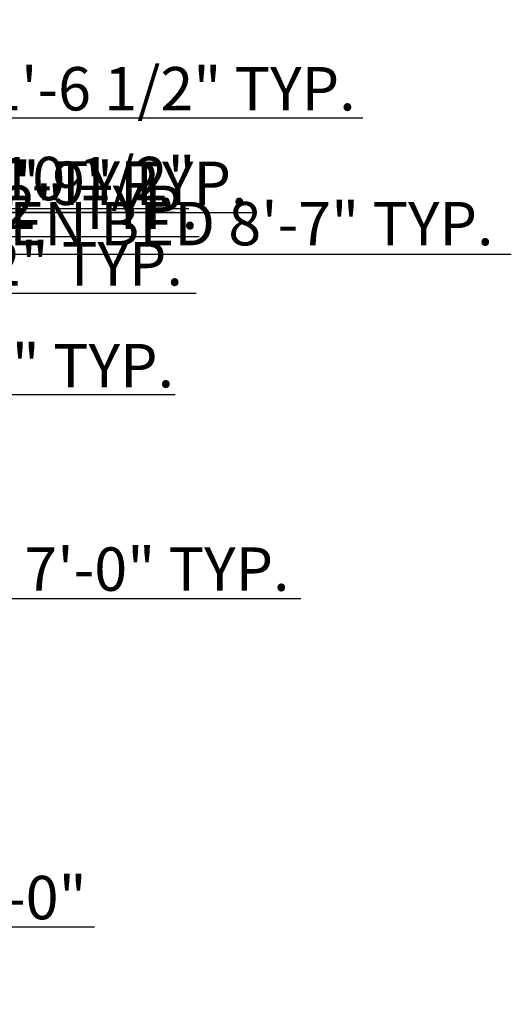
# Model space of a CAD drawing. Units: inches. Extents: x 830 to 1639, y 2591 to 3595.
# Tile 6 of 7: x 1367 to 1639, y 2716 to 3260. Entities that reach past the tile are written whole.
import ezdxf

# ---------------------------------------------------------------- set-up
doc = ezdxf.new("R2010")
doc.units = ezdxf.units.IN
doc.layers.add('A-ANNO-DIMS', color=2, linetype='Continuous', lineweight=18)
doc.styles.get("Standard").update_dxf_attribs({"font": 'arial.ttf'})
doc.dimstyles.new('ISO-25', dxfattribs={"dimtxt": 24, "dimasz": 12, "dimexe": 1.25, "dimexo": 0.625, "dimtad": 1, "dimdec": 0, "dimlunit": 3, "dimtxsty": 'Standard', "dimcen": 2.5, "dimadec": 0, "dimazin": 0, "dimtfac": 1, "dimtdec": 0, "dimtmove": 0, "dimatfit": 3, "dimfxl": 1, "dimarcsym": 0})

# ---------------------------------------------------------------- blocks, each defined once
blk = doc.blocks.new('*D23')
at = {"layer": 'A-ANNO-DIMS', "color": 0, "lineweight": -2, "transparency": 16777216}
for p, q in [((1272.59, 3057.79), (1272.59, 3051.77)), ((1281.59, 3057.79), (1281.59, 3051.77)), ((1260.59, 3053.02), (1248.59, 3053.02)), ((1272.59, 3053.02), (1281.59, 3053.02)), ((1293.59, 3053.02), (1453.13, 3053.02))]:
    blk.add_line(p, q, dxfattribs=at)
at = {"layer": 'A-ANNO-DIMS', "color": 0, "transparency": 16777216}
for points in [[(1260.59, 3055.02), (1260.59, 3051.02), (1272.59, 3053.02)], [(1293.59, 3055.02), (1293.59, 3051.02), (1281.59, 3053.02)]]:
    blk.add_solid(points, dxfattribs=at)
at = {"layer": 'Defpoints', "color": 0, "transparency": 16777216}
for p in [(1272.59, 3058.42), (1281.59, 3058.42), (1281.59, 3053.02)]:
    blk.add_point(p, dxfattribs=at)
at = {"layer": 'A-ANNO-DIMS', "color": 0, "transparency": 16777216, "insert": (1379.36, 3065.9), "char_height": 24, "attachment_point": 5}
blk.add_mtext('0\'-9" TYP.', dxfattribs=at)
blk = doc.blocks.new('*D25')
at = {"layer": 'A-ANNO-DIMS', "color": 0, "lineweight": -2, "transparency": 16777216}
for p, q in [((1272.59, 3156.83), (1272.59, 3152.6)), ((1281.59, 3156.83), (1281.59, 3152.6)), ((1260.59, 3153.85), (1248.59, 3153.85)), ((1272.59, 3153.85), (1281.59, 3153.85)), ((1293.59, 3153.85), (1453.13, 3153.85))]:
    blk.add_line(p, q, dxfattribs=at)
at = {"layer": 'A-ANNO-DIMS', "color": 0, "transparency": 16777216}
for points in [[(1260.59, 3155.85), (1260.59, 3151.85), (1272.59, 3153.85)], [(1293.59, 3155.85), (1293.59, 3151.85), (1281.59, 3153.85)]]:
    blk.add_solid(points, dxfattribs=at)
at = {"layer": 'Defpoints', "color": 0, "transparency": 16777216}
for p in [(1272.59, 3157.45), (1281.59, 3157.45), (1281.59, 3153.85)]:
    blk.add_point(p, dxfattribs=at)
at = {"layer": 'A-ANNO-DIMS', "color": 0, "transparency": 16777216, "insert": (1379.36, 3166.73), "char_height": 24, "attachment_point": 5}
blk.add_mtext('0\'-9" TYP.', dxfattribs=at)
blk = doc.blocks.new('*D26')
at = {"layer": 'A-ANNO-DIMS', "color": 0, "lineweight": -2, "transparency": 16777216}
for p, q in [((990.59, 3111.63), (990.59, 3107.9)), ((1011.31, 3111.63), (1011.31, 3107.9)), ((978.59, 3109.15), (966.59, 3109.15)), ((990.59, 3109.15), (1011.31, 3109.15)), ((1023.31, 3109.15), (1464.86, 3109.15))]:
    blk.add_line(p, q, dxfattribs=at)
at = {"layer": 'A-ANNO-DIMS', "color": 0, "transparency": 16777216}
for points in [[(978.59, 3111.15), (978.59, 3107.15), (990.59, 3109.15)], [(1023.31, 3111.15), (1023.31, 3107.15), (1011.31, 3109.15)]]:
    blk.add_solid(points, dxfattribs=at)
at = {"layer": 'Defpoints', "color": 0, "transparency": 16777216}
for p in [(990.59, 3112.26), (1011.31, 3112.26), (1011.31, 3109.15)]:
    blk.add_point(p, dxfattribs=at)
at = {"layer": 'A-ANNO-DIMS', "color": 0, "transparency": 16777216, "insert": (1250.08, 3122.18), "char_height": 24, "attachment_point": 5}
blk.add_mtext('NIGHTSTAND 1\'-8 1/2" TYP.', dxfattribs=at)
blk = doc.blocks.new('*D28')
at = {"layer": 'A-ANNO-DIMS', "color": 0, "lineweight": -2, "transparency": 16777216}
for p, q in [((1178.57, 2952.46), (1178.57, 2939.24)), ((1262.57, 2952.46), (1262.57, 2939.24)), ((1190.57, 2940.49), (1250.57, 2940.49)), ((1262.57, 2940.49), (1522.6, 2940.49))]:
    blk.add_line(p, q, dxfattribs=at)
at = {"layer": 'A-ANNO-DIMS', "color": 0, "transparency": 16777216}
for points in [[(1190.57, 2942.49), (1190.57, 2938.49), (1178.57, 2940.49)], [(1250.57, 2942.49), (1250.57, 2938.49), (1262.57, 2940.49)]]:
    blk.add_solid(points, dxfattribs=at)
at = {"layer": 'Defpoints', "color": 0, "transparency": 16777216}
for p in [(1178.57, 2953.09), (1262.57, 2953.09), (1262.57, 2940.49)]:
    blk.add_point(p, dxfattribs=at)
at = {"layer": 'A-ANNO-DIMS', "color": 0, "transparency": 16777216, "insert": (1398.58, 2953.53), "char_height": 24, "attachment_point": 5}
blk.add_mtext('SOFA 7\'-0" TYP.', dxfattribs=at)
blk = doc.blocks.new('*D30')
at = {"layer": 'A-ANNO-DIMS', "color": 0, "lineweight": -2, "transparency": 16777216}
for p, q in [((1239.54, 3157.95), (1239.54, 3152.37)), ((1272.59, 3157.95), (1272.59, 3152.37)), ((1251.54, 3153.62), (1260.59, 3153.62)), ((1272.59, 3153.62), (1498.29, 3153.62))]:
    blk.add_line(p, q, dxfattribs=at)
at = {"layer": 'A-ANNO-DIMS', "color": 0, "transparency": 16777216}
for points in [[(1251.54, 3155.62), (1251.54, 3151.62), (1239.54, 3153.62)], [(1260.59, 3155.62), (1260.59, 3151.62), (1272.59, 3153.62)]]:
    blk.add_solid(points, dxfattribs=at)
at = {"layer": 'Defpoints', "color": 0, "transparency": 16777216}
for p in [(1239.54, 3158.58), (1272.59, 3158.58), (1272.59, 3153.62)]:
    blk.add_point(p, dxfattribs=at)
at = {"layer": 'A-ANNO-DIMS', "color": 0, "transparency": 16777216, "insert": (1391.44, 3166.66), "char_height": 24, "attachment_point": 5}
blk.add_mtext('WC 2\'-9" TYP.', dxfattribs=at)
blk = doc.blocks.new('*D34')
at = {"layer": 'A-ANNO-DIMS', "color": 0, "lineweight": -2, "transparency": 16777216}
for p, q in [((1189.9, 3205.85), (1177.9, 3205.85)), ((1201.9, 3203.69), (1201.9, 3207.1)), ((1201.9, 3205.85), (1220.46, 3205.85)), ((1220.46, 3203.69), (1220.46, 3207.1)), ((1232.46, 3205.85), (1556.8, 3205.85))]:
    blk.add_line(p, q, dxfattribs=at)
at = {"layer": 'A-ANNO-DIMS', "color": 0, "transparency": 16777216}
for points in [[(1189.9, 3207.85), (1189.9, 3203.85), (1201.9, 3205.85)], [(1232.46, 3207.85), (1232.46, 3203.85), (1220.46, 3205.85)]]:
    blk.add_solid(points, dxfattribs=at)
at = {"layer": 'Defpoints', "color": 0, "transparency": 16777216}
for p in [(1220.46, 3205.85), (1201.9, 3203.07), (1220.46, 3203.07)]:
    blk.add_point(p, dxfattribs=at)
at = {"layer": 'A-ANNO-DIMS', "color": 0, "transparency": 16777216, "insert": (1400.63, 3218.88), "char_height": 24, "attachment_point": 5}
blk.add_mtext('BASIN 1\'-6 1/2" TYP.', dxfattribs=at)
blk = doc.blocks.new('*D36')
at = {"layer": 'A-ANNO-DIMS', "color": 0, "lineweight": -2, "transparency": 16777216}
for p, q in [((1169.49, 3115.77), (1169.49, 3131.86)), ((1181.49, 3130.61), (1260.59, 3130.61)), ((1272.59, 3115.77), (1272.59, 3131.86)), ((1272.59, 3130.61), (1638.88, 3130.61))]:
    blk.add_line(p, q, dxfattribs=at)
at = {"layer": 'A-ANNO-DIMS', "color": 0, "transparency": 16777216}
for points in [[(1181.49, 3132.61), (1181.49, 3128.61), (1169.49, 3130.61)], [(1260.59, 3132.61), (1260.59, 3128.61), (1272.59, 3130.61)]]:
    blk.add_solid(points, dxfattribs=at)
at = {"layer": 'Defpoints', "color": 0, "transparency": 16777216}
for p in [(1272.59, 3130.61), (1169.49, 3115.15), (1272.59, 3115.15)]:
    blk.add_point(p, dxfattribs=at)
at = {"layer": 'A-ANNO-DIMS', "color": 0, "transparency": 16777216, "insert": (1461.74, 3144.38), "char_height": 24, "attachment_point": 5}
blk.add_mtext('QUEEN BED 8\'-7" TYP.', dxfattribs=at)
blk = doc.blocks.new('*D39')
at = {"layer": 'A-ANNO-DIMS', "color": 0, "lineweight": -2, "transparency": 16777216}
for p, q in [((1197.62, 3140.39), (1185.62, 3140.39)), ((1209.62, 3142.46), (1209.62, 3139.14)), ((1209.62, 3140.39), (1220.27, 3140.39)), ((1220.27, 3142.46), (1220.27, 3139.14)), ((1232.27, 3140.39), (1466.38, 3140.39))]:
    blk.add_line(p, q, dxfattribs=at)
at = {"layer": 'A-ANNO-DIMS', "color": 0, "transparency": 16777216}
for points in [[(1197.62, 3142.39), (1197.62, 3138.39), (1209.62, 3140.39)], [(1232.27, 3142.39), (1232.27, 3138.39), (1220.27, 3140.39)]]:
    blk.add_solid(points, dxfattribs=at)
at = {"layer": 'Defpoints', "color": 0, "transparency": 16777216}
for p in [(1209.62, 3143.09), (1220.27, 3143.09), (1220.27, 3140.39)]:
    blk.add_point(p, dxfattribs=at)
at = {"layer": 'A-ANNO-DIMS', "color": 0, "transparency": 16777216, "insert": (1355.32, 3153.43), "char_height": 24, "attachment_point": 5}
blk.add_mtext('0\'-10 1/2" TYP.', dxfattribs=at)
blk = doc.blocks.new('*D42')
at = {"layer": 'A-ANNO-DIMS', "color": 0, "lineweight": -2, "transparency": 16777216}
for p, q in [((1062.05, 2763.79), (1062.05, 2757.77)), ((1098.05, 2763.79), (1098.05, 2757.77)), ((1074.05, 2759.02), (1086.05, 2759.02)), ((1098.05, 2759.02), (1408.67, 2759.02))]:
    blk.add_line(p, q, dxfattribs=at)
at = {"layer": 'A-ANNO-DIMS', "color": 0, "transparency": 16777216}
for points in [[(1074.05, 2761.02), (1074.05, 2757.02), (1062.05, 2759.02)], [(1086.05, 2761.02), (1086.05, 2757.02), (1098.05, 2759.02)]]:
    blk.add_solid(points, dxfattribs=at)
at = {"layer": 'Defpoints', "color": 0, "transparency": 16777216}
for p in [(1062.05, 2764.42), (1098.05, 2764.42), (1098.05, 2759.02)]:
    blk.add_point(p, dxfattribs=at)
at = {"layer": 'A-ANNO-DIMS', "color": 0, "transparency": 16777216, "insert": (1259.36, 2772.07), "char_height": 24, "attachment_point": 5}
blk.add_mtext('DOUBLE SINK 3\'-0"', dxfattribs=at)
blk = doc.blocks.new('*D77')
at = {"layer": 'A-ANNO-DIMS', "color": 0, "lineweight": -2, "transparency": 16777216}
for p, q in [((1197.62, 3155.72), (1185.62, 3155.72)), ((1209.62, 3155.72), (1220.27, 3155.72)), ((1460.7, 3155.7), (1232.27, 3155.72))]:
    blk.add_line(p, q, dxfattribs=at)
at = {"layer": 'A-ANNO-DIMS', "color": 0, "transparency": 16777216}
for points in [[(1197.62, 3157.72), (1197.62, 3153.72), (1209.62, 3155.72)], [(1232.27, 3157.72), (1232.27, 3153.72), (1220.27, 3155.72)]]:
    blk.add_solid(points, dxfattribs=at)
at = {"layer": 'Defpoints', "color": 0, "transparency": 16777216}
for p in [(1209.62, 3155.72), (1220.27, 3155.72)]:
    blk.add_point(p, dxfattribs=at)
at = {"layer": 'A-ANNO-DIMS', "color": 0, "transparency": 16777216, "insert": (1352.48, 3169.26), "char_height": 24, "attachment_point": 5, "rotation": 359.9951}
blk.add_mtext('2X ∅0\'-10 1/2"', dxfattribs=at)

msp = doc.modelspace()

# ---------------------------------------------------------------- dimensions: what is measured, and where the dimension line sits
at = {"layer": 'A-ANNO-DIMS'}
for base, p1, p2, text, picture, middle in [((1220.46, 3205.85), (1201.9, 3203.07), (1220.46, 3203.07), 'BASIN <> TYP.', '*D34', (1400.63, 3218.88)), ((1272.59, 3130.61), (1169.49, 3115.15), (1272.59, 3115.15), 'QUEEN BED <> TYP.', '*D36', (1461.74, 3144.38)), ((1272.5897, 3153.6208), (1239.5435, 3158.5777), (1272.5897, 3158.5777), 'WC <> TYP.', '*D30', (1391.4384, 3166.6551)), ((1220.2661, 3140.394), (1209.616, 3143.0874), (1220.2661, 3143.0874), '<> TYP.', '*D39', (1355.3222, 3153.4283)), ((1281.59, 3153.85), (1272.59, 3157.45), (1281.59, 3157.45), '<> TYP.', '*D25', (1379.36, 3166.73)), ((1011.31, 3109.15), (990.59, 3112.26), (1011.31, 3112.26), 'NIGHTSTAND <> TYP.', '*D26', (1250.08, 3122.18)), ((1281.59, 3053.02), (1272.59, 3058.42), (1281.59, 3058.42), '<> TYP.', '*D23', (1379.36, 3065.9)), ((1262.57, 2940.49), (1178.57, 2953.09), (1262.57, 2953.09), 'SOFA <> TYP.', '*D28', (1398.58, 2953.53)), ((1098.05, 2759.02), (1062.05, 2764.42), (1098.05, 2764.42), 'DOUBLE SINK <>', '*D42', (1259.36, 2772.07))]:
    dim = msp.add_linear_dim(base=base, p1=p1, p2=p2, text=text, dimstyle='ISO-25', override={"dimdec": 1, "dimlfac": 1, "dimrnd": 0, "dimzin": 1, "dimdsep": 46, "dimlunit": 4, "dimfrac": 2}, dxfattribs=at)
    dim.commit()
    dim.dimension.update_dxf_attribs({"geometry": picture, "text_midpoint": middle})
dim = msp.add_diameter_dim_2p(p1=(1209.616, 3155.7189), p2=(1220.2661, 3155.718), text='2X <>', dimstyle='ISO-25', override={"dimdec": 1, "dimlfac": 1, "dimrnd": 0, "dimzin": 1, "dimdsep": 46, "dimlunit": 4, "dimfrac": 2}, dxfattribs=at)
dim.commit()
dim.dimension.update_dxf_attribs({"geometry": '*D77', "text_midpoint": (1352.4818, 3155.7068)})

doc.saveas('drawing.dxf')
